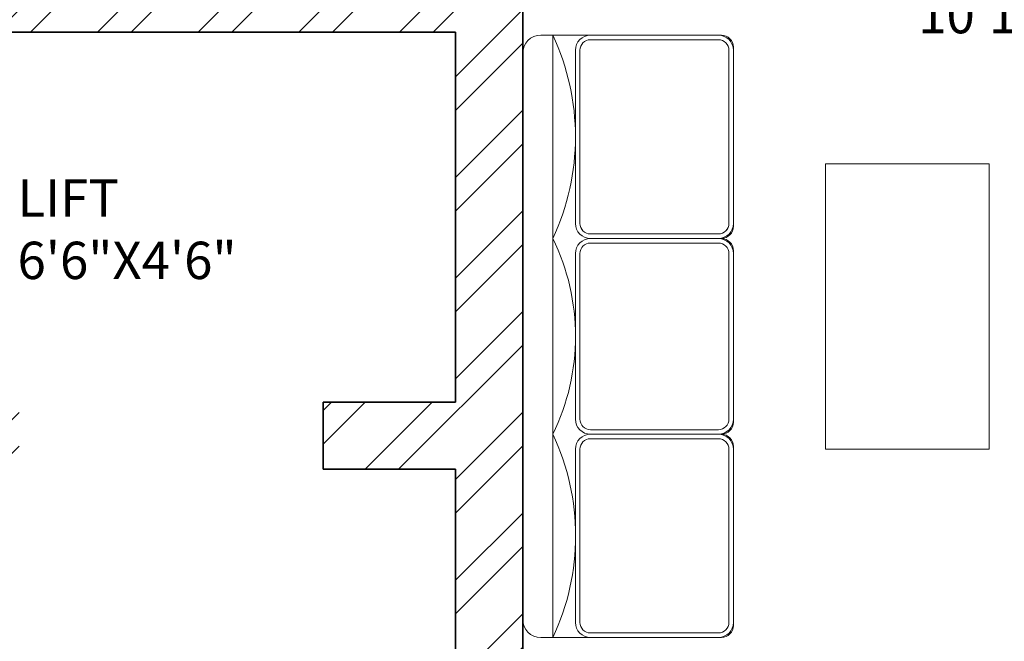
# Model space of a CAD drawing. Units: inches. Extents: x 2120 to 4013, y 1390 to 3019.
# Tile 36 of 59: x 2657 to 2789, y 2048 to 2131. Entities that reach past the tile are written whole.
import ezdxf

# ---------------------------------------------------------------- set-up
doc = ezdxf.new("R2010")
doc.units = ezdxf.units.IN
for name, color, linetype, lineweight in [('A-AREA-IDEN', 7, 'Continuous', 18), ('A-FURN', 8, 'Continuous', 13), ('A-WALL', 7, 'Continuous', 35), ('A-WALL-PATT', 252, 'Continuous', 13)]:
    doc.layers.add(name, color=color, linetype=linetype, lineweight=lineweight)
doc.styles.get("Standard").update_dxf_attribs({"font": 'arial.ttf'})

# ---------------------------------------------------------------- blocks, each defined once
blk = doc.blocks.new('TABLE-COFFEE')
blk.add_lwpolyline([(0, 38.19), (21.88, 38.19), (21.88, 0), (0, 0)], close=True)

msp = doc.modelspace()

# ---------------------------------------------------------------- hatches: boundary and pattern name
at = {"layer": 'A-WALL-PATT'}
h = msp.add_hatch(dxfattribs=at)
h.set_pattern_fill('ANSI32', color=256)
h.paths.add_polyline_path([(2271.7331, 2343.531), (2283.3788, 2343.531), (2283.3788, 2348.031), (2283.3788, 2352.5306), (2262.7331, 2352.5306), (2262.7331, 2182.638), (2267.2331, 2182.638), (2271.7331, 2182.638), (2271.7331, 2219.031), (2391.7331, 2219.031), (2391.7331, 2214.189), (2393.9831, 2214.189), (2396.2331, 2214.189), (2396.2331, 2219.031), (2420.2331, 2219.031), (2420.2331, 2225.7535), (2417.2197, 2225.7535), (2415.7331, 2225.7535), (2415.7331, 2223.5306), (2271.7331, 2223.5306)])
h.paths.add_polyline_path([(2380.0942, 2352.5306), (2343.3788, 2352.5306), (2343.3788, 2343.531), (2363.2331, 2343.531), (2363.2331, 2288.8489), (2365.4831, 2288.8489), (2367.7331, 2288.8489), (2367.7331, 2343.531), (2380.0942, 2343.531)], flags=17)
h.paths.add_polyline_path([(2432.4339, 2352.5306), (2404.0943, 2352.5306), (2404.0943, 2343.531), (2415.7331, 2343.531), (2415.7331, 2264.0306), (2367.7331, 2264.0306), (2367.7331, 2266.4872), (2363.2331, 2266.4872), (2363.2331, 2259.531), (2367.7331, 2259.531), (2415.7331, 2259.531), (2415.7331, 2255.0658), (2420.2331, 2255.0658), (2420.2331, 2259.531), (2424.5717, 2259.531), (2424.5717, 2261.781), (2424.5717, 2264.0306), (2420.2331, 2264.0306), (2420.2331, 2343.531), (2432.4339, 2343.531)])
h.paths.add_polyline_path([(2508.9115, 2352.5306), (2456.4339, 2352.5306), (2456.4339, 2343.531), (2468.2331, 2343.531), (2468.2331, 2264.0306), (2448.0487, 2264.0306), (2448.0487, 2259.531), (2468.2331, 2259.531), (2468.2331, 2255.5496), (2472.7331, 2255.5496), (2472.7331, 2343.531), (2508.9115, 2343.531)])
h.paths.add_polyline_path([(2637.7331, 2352.5306), (2544.9116, 2352.5306), (2544.9116, 2343.531), (2589.7331, 2343.531), (2633.2331, 2343.531), (2637.7331, 2343.531)])
h.paths.add_polyline_path([(2594.2331, 2343.5306), (2589.7331, 2343.5306), (2589.7331, 2259.5306), (2589.7331, 2252.4915), (2591.9831, 2252.4915), (2594.2331, 2252.4915)])
h.paths.add_polyline_path([(2637.7331, 2223.5306), (2594.2331, 2223.5306), (2594.2331, 2230.1988), (2591.9831, 2230.1988), (2589.7331, 2230.1988), (2589.7331, 2223.5306), (2472.7331, 2223.5306), (2468.2331, 2223.5306), (2468.2331, 2219.031), (2628.7331, 2219.031), (2628.7331, 2138.031), (2637.7331, 2138.031)])
h.paths.add_polyline_path([(3822.6535, 2458.4402), (3874.9468, 2458.4402), (3874.9468, 2476.9866), (3822.6535, 2476.9866)], flags=9)
h.paths.add_polyline_path([(3834.6921, 2781.8174), (3935.9206, 2781.8174), (3935.9206, 2800.3638), (3834.6921, 2800.3638)], flags=9)
h.paths.add_polyline_path([(3832.2843, 2837.9683), (3884.5776, 2837.9683), (3884.5776, 2856.5146), (3832.2843, 2856.5146)], flags=9)
h.paths.add_polyline_path([(3830.9388, 2861.4782), (3956.8958, 2861.4782), (3956.8958, 2880.0245), (3830.9388, 2880.0245)], flags=9)
h.paths.add_polyline_path([(3870.6966, 2352.5752), (3887.9272, 2352.5752), (3887.9272, 2377.3037), (3870.6966, 2377.3037)], flags=9)
h.paths.add_polyline_path([(3289.2701, 2413.161), (3435.2223, 2413.161), (3435.2223, 2450.2538), (3289.2701, 2450.2538)], flags=9)
h.paths.add_polyline_path([(2487.6944, 2414.3601), (2637.8335, 2414.3601), (2637.8335, 2451.4528), (2487.6944, 2451.4528)], flags=9)
h.paths.add_polyline_path([(2567.3724, 1457.9199), (2815.296, 1457.9199), (2815.296, 1495.0127), (2567.3724, 1495.0127)], flags=9)
h.paths.add_polyline_path([(2655.3825, 2093.2363), (2685.9555, 2093.2363), (2685.9555, 2111.8937), (2655.3825, 2111.8937)], flags=9)
h.paths.add_polyline_path([(2543.9218, 1550.6671), (2587.8406, 1550.6671), (2587.8406, 1569.3244), (2543.9218, 1569.3244)], flags=9)
h.paths.add_polyline_path([(2905.1384, 1543.8113), (2949.0572, 1543.8113), (2949.0572, 1562.4686), (2905.1384, 1562.4686)], flags=9)
h.paths.add_polyline_path([(2736.4118, 1702.4736), (2784.2153, 1702.4736), (2784.2153, 1721.1309), (2736.4118, 1721.1309)], flags=9)
h.paths.add_polyline_path([(2912.8666, 1710.4168), (2951.707, 1710.4168), (2951.707, 1729.0741), (2912.8666, 1729.0741)], flags=9)
h.paths.add_polyline_path([(2923.5785, 1763.5038), (2959.7279, 1763.5038), (2959.7279, 1782.1611), (2923.5785, 1782.1611)], flags=9)
h.paths.add_polyline_path([(2925.2114, 1809.6137), (2967.1861, 1809.6137), (2967.1861, 1828.271), (2925.2114, 1828.271)], flags=9)
h.paths.add_polyline_path([(2996.2711, 1878.9003), (2996.2711, 1913.109), (2977.6138, 1913.109), (2977.6138, 1878.9003)], flags=9)
h.paths.add_polyline_path([(2883.0859, 1895.7192), (2927.1855, 1895.7192), (2927.1855, 1914.3766), (2883.0859, 1914.3766)], flags=9)
h.paths.add_polyline_path([(2787.3924, 1810.8013), (2841.0213, 1810.8013), (2841.0213, 1829.4587), (2787.3924, 1829.4587)], flags=9)
h.paths.add_polyline_path([(2775.6399, 2101.7395), (2829.2689, 2101.7395), (2829.2689, 2120.3968), (2775.6399, 2120.3968)], flags=9)
h.paths.add_polyline_path([(2913.0263, 2075.817), (2951.8667, 2075.817), (2951.8667, 2094.4744), (2913.0263, 2094.4744)], flags=9)
h.paths.add_polyline_path([(2929.966, 2133.3669), (2966.1154, 2133.3669), (2966.1154, 2152.0243), (2929.966, 2152.0243)], flags=9)
h.paths.add_polyline_path([(2932.7502, 2182.6088), (2968.8996, 2182.6088), (2968.8996, 2201.2662), (2932.7502, 2201.2662)], flags=9)
h.paths.add_polyline_path([(2996.0681, 2266.3173), (2996.0681, 2300.5261), (2977.4108, 2300.5261), (2977.4108, 2266.3173)], flags=9)
h.paths.add_polyline_path([(2885.1039, 2279.2186), (2929.2035, 2279.2186), (2929.2035, 2297.8759), (2885.1039, 2297.8759)], flags=9)
h.paths.add_polyline_path([(2735.7042, 2218.3197), (2783.5078, 2218.3197), (2783.5078, 2236.9771), (2735.7042, 2236.9771)], flags=9)
h.paths.add_polyline_path([(2635.6049, 2044.0085), (2648.9678, 2044.0085), (2648.9678, 2054.312), (2635.6049, 2054.312)], flags=9)
h.paths.add_polyline_path([(2714.0148, 1923.0473), (2727.3777, 1923.0473), (2727.3777, 1933.3508), (2714.0148, 1933.3508)], flags=9)
h.paths.add_polyline_path([(2709.0345, 1988.1628), (2722.3974, 1988.1628), (2722.3974, 1998.4663), (2709.0345, 1998.4663)], flags=9)
h.paths.add_polyline_path([(2592.8935, 1962.1763), (2606.2564, 1962.1763), (2606.2564, 1972.4799), (2592.8935, 1972.4799)], flags=9)
h.paths.add_polyline_path([(2618.3996, 1985.9724), (2644.1942, 1985.9724), (2644.1942, 1996.2759), (2618.3996, 1996.2759)], flags=9)
h.paths.add_polyline_path([(2601.279, 1920.5869), (2614.6419, 1920.5869), (2614.6419, 1930.8904), (2601.279, 1930.8904)], flags=9)
h.paths.add_polyline_path([(2692.3278, 1932.7645), (2704.5311, 1932.7645), (2704.5311, 1943.0681), (2692.3278, 1943.0681)], flags=9)
h.paths.add_polyline_path([(2311.122, 1672.7318), (2355.0408, 1672.7318), (2355.0408, 1691.3892), (2311.122, 1691.3892)], flags=9)
h.paths.add_polyline_path([(2456.2551, 1632.3198), (2492.4796, 1632.3198), (2492.4796, 1650.9772), (2456.2551, 1650.9772)], flags=9)
h.paths.add_polyline_path([(2401.0766, 1631.4793), (2437.301, 1631.4793), (2437.301, 1650.1367), (2401.0766, 1650.1367)], flags=9)
h.paths.add_polyline_path([(2546.7054, 1700.9235), (2594.509, 1700.9235), (2594.509, 1719.5809), (2546.7054, 1719.5809)], flags=9)
h.paths.add_polyline_path([(2445.4866, 1766.9937), (2497.5261, 1766.9937), (2497.5261, 1785.651), (2445.4866, 1785.651)], flags=9)
h.paths.add_polyline_path([(2287.9992, 1739.7675), (2326.8396, 1739.7675), (2326.8396, 1758.4248), (2287.9992, 1758.4248)], flags=9)
h.paths.add_polyline_path([(2458.5279, 1924.7607), (2510.5675, 1924.7607), (2510.5675, 1943.4181), (2458.5279, 1943.4181)], flags=9)
h.paths.add_polyline_path([(2309.2811, 1902.7642), (2345.4305, 1902.7642), (2345.4305, 1921.4215), (2309.2811, 1921.4215)], flags=9)
h.paths.add_polyline_path([(2490.7554, 2018.9392), (2530.7896, 2018.9392), (2530.7896, 2037.5965), (2490.7554, 2037.5965)], flags=9)
h.paths.add_polyline_path([(2402.143, 2024.7393), (2438.5414, 2024.7393), (2438.5414, 2043.3966), (2402.143, 2043.3966)], flags=9)
h.paths.add_polyline_path([(2287.856, 1931.7926), (2326.6964, 1931.7926), (2326.6964, 1950.4499), (2287.856, 1950.4499)], flags=9)
h.paths.add_polyline_path([(2281.7979, 2193.5771), (2320.6383, 2193.5771), (2320.6383, 2212.2344), (2281.7979, 2212.2344)], flags=25)
h.paths.add_polyline_path([(2484.0754, 2093.892), (2536.115, 2093.892), (2536.115, 2112.5494), (2484.0754, 2112.5494)], flags=9)
h.paths.add_polyline_path([(2624.7948, 2281.8639), (2624.7948, 2311.4137), (2606.1375, 2311.4137), (2606.1375, 2281.8639)], flags=9)
h.paths.add_polyline_path([(2507.5036, 2290.3639), (2541.934, 2290.3639), (2541.934, 2309.0212), (2507.5036, 2309.0212)], flags=9)
h.paths.add_polyline_path([(2423.1076, 2285.2202), (2459.332, 2285.2202), (2459.332, 2303.8776), (2423.1076, 2303.8776)], flags=9)
h.paths.add_polyline_path([(2374.5467, 2289.6272), (2410.7711, 2289.6272), (2410.7711, 2308.2846), (2374.5467, 2308.2846)], flags=25)
h.paths.add_polyline_path([(2277.4907, 2227.5651), (2316.3311, 2227.5651), (2316.3311, 2246.2224), (2277.4907, 2246.2224)], flags=25)
h.paths.add_polyline_path([(2655.3825, 2093.2367), (2685.9555, 2093.2367), (2685.9555, 2111.894), (2655.3825, 2111.894)], flags=9)
h.paths.add_polyline_path([(2543.9217, 1550.6674), (2587.8406, 1550.6674), (2587.8406, 1569.3247), (2543.9217, 1569.3247)], flags=9)
h.paths.add_polyline_path([(2905.1384, 1543.8116), (2949.0572, 1543.8116), (2949.0572, 1562.4689), (2905.1384, 1562.4689)], flags=9)
h.paths.add_polyline_path([(2736.4118, 1702.4739), (2784.2153, 1702.4739), (2784.2153, 1721.1312), (2736.4118, 1721.1312)], flags=9)
h.paths.add_polyline_path([(2912.8666, 1710.4171), (2951.707, 1710.4171), (2951.707, 1729.0744), (2912.8666, 1729.0744)], flags=9)
h.paths.add_polyline_path([(2923.5785, 1763.5041), (2959.7279, 1763.5041), (2959.7279, 1782.1614), (2923.5785, 1782.1614)], flags=9)
h.paths.add_polyline_path([(2925.2114, 1809.614), (2967.1861, 1809.614), (2967.1861, 1828.2713), (2925.2114, 1828.2713)], flags=9)
h.paths.add_polyline_path([(2996.2711, 1878.9006), (2996.2711, 1913.1094), (2977.6137, 1913.1094), (2977.6137, 1878.9006)], flags=9)
h.paths.add_polyline_path([(2883.0859, 1895.7195), (2927.1855, 1895.7195), (2927.1855, 1914.3769), (2883.0859, 1914.3769)], flags=9)
h.paths.add_polyline_path([(2787.3924, 1810.8016), (2841.0213, 1810.8016), (2841.0213, 1829.459), (2787.3924, 1829.459)], flags=9)
h.paths.add_polyline_path([(2775.6399, 2101.7398), (2829.2688, 2101.7398), (2829.2688, 2120.3971), (2775.6399, 2120.3971)], flags=9)
h.paths.add_polyline_path([(2913.0263, 2075.8173), (2951.8667, 2075.8173), (2951.8667, 2094.4747), (2913.0263, 2094.4747)], flags=9)
h.paths.add_polyline_path([(2929.966, 2133.3672), (2966.1154, 2133.3672), (2966.1154, 2152.0246), (2929.966, 2152.0246)], flags=9)
h.paths.add_polyline_path([(2932.7502, 2182.6091), (2968.8996, 2182.6091), (2968.8996, 2201.2665), (2932.7502, 2201.2665)], flags=9)
h.paths.add_polyline_path([(2996.0681, 2266.3176), (2996.0681, 2300.5264), (2977.4108, 2300.5264), (2977.4108, 2266.3176)], flags=9)
h.paths.add_polyline_path([(2885.1039, 2279.2189), (2929.2035, 2279.2189), (2929.2035, 2297.8762), (2885.1039, 2297.8762)], flags=9)
h.paths.add_polyline_path([(2735.7042, 2218.32), (2783.5078, 2218.32), (2783.5078, 2236.9774), (2735.7042, 2236.9774)], flags=9)
h.paths.add_polyline_path([(2635.6048, 2044.0088), (2648.9677, 2044.0088), (2648.9677, 2054.3123), (2635.6048, 2054.3123)], flags=9)
h.paths.add_polyline_path([(2714.0148, 1923.0476), (2727.3777, 1923.0476), (2727.3777, 1933.3511), (2714.0148, 1933.3511)], flags=9)
h.paths.add_polyline_path([(2709.0345, 1988.1631), (2722.3974, 1988.1631), (2722.3974, 1998.4666), (2709.0345, 1998.4666)], flags=9)
h.paths.add_polyline_path([(2592.8935, 1962.1766), (2606.2564, 1962.1766), (2606.2564, 1972.4802), (2592.8935, 1972.4802)], flags=9)
h.paths.add_polyline_path([(2618.3995, 1985.9727), (2644.1942, 1985.9727), (2644.1942, 1996.2762), (2618.3995, 1996.2762)], flags=9)
h.paths.add_polyline_path([(2601.279, 1920.5872), (2614.6419, 1920.5872), (2614.6419, 1930.8908), (2601.279, 1930.8908)], flags=9)
h.paths.add_polyline_path([(2692.3278, 1932.7648), (2704.5311, 1932.7648), (2704.5311, 1943.0684), (2692.3278, 1943.0684)], flags=9)
h.paths.add_polyline_path([(2311.122, 1672.7321), (2355.0408, 1672.7321), (2355.0408, 1691.3895), (2311.122, 1691.3895)], flags=9)
h.paths.add_polyline_path([(2456.2551, 1632.3201), (2492.4795, 1632.3201), (2492.4795, 1650.9775), (2456.2551, 1650.9775)], flags=9)
h.paths.add_polyline_path([(2401.0766, 1631.4796), (2437.301, 1631.4796), (2437.301, 1650.137), (2401.0766, 1650.137)], flags=9)
h.paths.add_polyline_path([(2546.7054, 1700.9238), (2594.509, 1700.9238), (2594.509, 1719.5812), (2546.7054, 1719.5812)], flags=9)
h.paths.add_polyline_path([(2445.4866, 1766.994), (2497.5261, 1766.994), (2497.5261, 1785.6513), (2445.4866, 1785.6513)], flags=9)
h.paths.add_polyline_path([(2287.9992, 1739.7678), (2326.8396, 1739.7678), (2326.8396, 1758.4251), (2287.9992, 1758.4251)], flags=9)
h.paths.add_polyline_path([(2458.5279, 1924.7611), (2510.5675, 1924.7611), (2510.5675, 1943.4184), (2458.5279, 1943.4184)], flags=9)
h.paths.add_polyline_path([(2309.2811, 1902.7645), (2345.4305, 1902.7645), (2345.4305, 1921.4218), (2309.2811, 1921.4218)], flags=9)
h.paths.add_polyline_path([(2490.7554, 2018.9395), (2530.7895, 2018.9395), (2530.7895, 2037.5968), (2490.7554, 2037.5968)], flags=9)
h.paths.add_polyline_path([(2402.143, 2024.7396), (2438.5413, 2024.7396), (2438.5413, 2043.3969), (2402.143, 2043.3969)], flags=9)
h.paths.add_polyline_path([(2287.856, 1931.7929), (2326.6964, 1931.7929), (2326.6964, 1950.4502), (2287.856, 1950.4502)], flags=9)
h.paths.add_polyline_path([(2281.7979, 2193.5774), (2320.6383, 2193.5774), (2320.6383, 2212.2347), (2281.7979, 2212.2347)], flags=25)
h.paths.add_polyline_path([(2484.0754, 2093.8924), (2536.115, 2093.8924), (2536.115, 2112.5497), (2484.0754, 2112.5497)], flags=9)
h.paths.add_polyline_path([(2624.7948, 2281.8642), (2624.7948, 2311.414), (2606.1374, 2311.414), (2606.1374, 2281.8642)], flags=9)
h.paths.add_polyline_path([(2507.5035, 2290.3642), (2541.934, 2290.3642), (2541.934, 2309.0215), (2507.5035, 2309.0215)], flags=9)
h.paths.add_polyline_path([(2423.1075, 2285.2205), (2459.332, 2285.2205), (2459.332, 2303.8779), (2423.1075, 2303.8779)], flags=9)
h.paths.add_polyline_path([(2374.5467, 2289.6275), (2410.7711, 2289.6275), (2410.7711, 2308.2849), (2374.5467, 2308.2849)], flags=25)
h.paths.add_polyline_path([(2277.4907, 2227.5654), (2316.3311, 2227.5654), (2316.3311, 2246.2227), (2277.4907, 2246.2227)], flags=25)
h = msp.add_hatch(dxfattribs=at)
h.set_pattern_fill('ANSI32', color=256)
h.paths.add_polyline_path([(2271.7331, 1980.389), (2262.7331, 1980.389), (2262.7331, 1912.8434), (2267.2331, 1912.8434), (2271.7331, 1912.8434), (2271.7331, 1922.531), (2351.2331, 1922.531), (2351.2331, 1901.4728), (2355.7331, 1901.4728), (2355.7331, 1922.531), (2357.9815, 1922.531), (2357.9815, 1926.5306), (2271.7331, 1926.5306)])
h.paths.add_polyline_path([(2589.2331, 1949.1622), (2584.7331, 1949.1622), (2580.2331, 1949.1622), (2580.2331, 1874.5306), (2355.7331, 1874.5306), (2355.7331, 1880.1922), (2351.2331, 1880.1922), (2351.2331, 1874.5306), (2271.7331, 1874.5306), (2271.7331, 1888.8431), (2262.7331, 1888.8431), (2262.7331, 1842.2909), (2267.2331, 1842.2909), (2271.7331, 1842.2909), (2271.7331, 1865.531), (2415.7331, 1865.531), (2415.7331, 1779.7286), (2420.2331, 1779.7286), (2420.2331, 1865.531), (2589.2331, 1865.531)])
h.paths.add_polyline_path([(2271.7331, 1782.2906), (2262.7331, 1782.2906), (2262.7331, 1711.4639), (2267.2331, 1711.4639), (2271.7331, 1711.4639), (2271.7331, 1738.031), (2420.2331, 1738.031), (2420.2331, 1742.531), (2420.2331, 1747.3376), (2417.9831, 1747.3376), (2415.7331, 1747.3376), (2415.7331, 1742.5306), (2271.7331, 1742.5306)])
h.paths.add_polyline_path([(2271.7331, 1627.031), (2362.3957, 1627.031), (2362.3957, 1629.281), (2362.3957, 1631.5306), (2271.7331, 1631.5306), (2271.7331, 1675.4636), (2262.7331, 1675.4636), (2262.7331, 1581.531), (2405.3032, 1581.531), (2405.3032, 1586.031), (2405.3032, 1590.5306), (2396.2331, 1590.5306), (2396.2331, 1691.4513), (2418.7206, 1691.4513), (2418.7206, 1695.951), (2396.2331, 1695.951), (2391.7331, 1695.951), (2391.7331, 1631.5306), (2386.7425, 1631.5306), (2386.7425, 1629.2806), (2386.7425, 1627.031), (2391.7331, 1627.031), (2391.7331, 1586.1709), (2271.7331, 1586.1709)])
h.paths.add_polyline_path([(2459.6703, 1590.5306), (2429.3032, 1590.5306), (2429.3032, 1581.531), (2459.6703, 1581.531), (2459.6703, 1586.031)])
h.paths.add_polyline_path([(2501.2331, 1590.531), (2501.2331, 1665.0195), (2498.9831, 1665.0195), (2496.7331, 1665.0195), (2496.7331, 1590.5306), (2483.8201, 1590.5306), (2483.8201, 1590.1579), (2483.6704, 1590.1579), (2483.6704, 1581.531), (2505.0196, 1581.531), (2505.0196, 1583.781), (2505.0196, 1586.0306), (2501.2331, 1586.0306)])
h.paths.add_polyline_path([(2544.1361, 1583.781), (2544.1361, 1586.0306), (2527.1368, 1586.0306), (2527.1368, 1583.7806), (2527.1368, 1581.531), (2544.1361, 1581.531)])
h.paths.add_polyline_path([(3822.6535, 2458.4402), (3874.9468, 2458.4402), (3874.9468, 2476.9866), (3822.6535, 2476.9866)], flags=9)
h.paths.add_polyline_path([(3834.6921, 2781.8174), (3935.9206, 2781.8174), (3935.9206, 2800.3638), (3834.6921, 2800.3638)], flags=9)
h.paths.add_polyline_path([(3832.2843, 2837.9683), (3884.5776, 2837.9683), (3884.5776, 2856.5146), (3832.2843, 2856.5146)], flags=9)
h.paths.add_polyline_path([(3830.9388, 2861.4782), (3956.8958, 2861.4782), (3956.8958, 2880.0245), (3830.9388, 2880.0245)], flags=9)
h.paths.add_polyline_path([(3870.6966, 2352.5752), (3887.9272, 2352.5752), (3887.9272, 2377.3037), (3870.6966, 2377.3037)], flags=9)
h.paths.add_polyline_path([(3289.2701, 2413.161), (3435.2223, 2413.161), (3435.2223, 2450.2538), (3289.2701, 2450.2538)], flags=9)
h.paths.add_polyline_path([(2487.6944, 2414.3601), (2637.8335, 2414.3601), (2637.8335, 2451.4528), (2487.6944, 2451.4528)], flags=9)
h.paths.add_polyline_path([(2567.3724, 1457.9199), (2815.296, 1457.9199), (2815.296, 1495.0127), (2567.3724, 1495.0127)], flags=9)
h.paths.add_polyline_path([(2655.3825, 2093.2363), (2685.9555, 2093.2363), (2685.9555, 2111.8937), (2655.3825, 2111.8937)], flags=9)
h.paths.add_polyline_path([(2543.9218, 1550.6671), (2587.8406, 1550.6671), (2587.8406, 1569.3244), (2543.9218, 1569.3244)], flags=9)
h.paths.add_polyline_path([(2905.1384, 1543.8113), (2949.0572, 1543.8113), (2949.0572, 1562.4686), (2905.1384, 1562.4686)], flags=9)
h.paths.add_polyline_path([(2736.4118, 1702.4736), (2784.2153, 1702.4736), (2784.2153, 1721.1309), (2736.4118, 1721.1309)], flags=9)
h.paths.add_polyline_path([(2912.8666, 1710.4168), (2951.707, 1710.4168), (2951.707, 1729.0741), (2912.8666, 1729.0741)], flags=9)
h.paths.add_polyline_path([(2923.5785, 1763.5038), (2959.7279, 1763.5038), (2959.7279, 1782.1611), (2923.5785, 1782.1611)], flags=9)
h.paths.add_polyline_path([(2925.2114, 1809.6137), (2967.1861, 1809.6137), (2967.1861, 1828.271), (2925.2114, 1828.271)], flags=9)
h.paths.add_polyline_path([(2996.2711, 1878.9003), (2996.2711, 1913.109), (2977.6138, 1913.109), (2977.6138, 1878.9003)], flags=9)
h.paths.add_polyline_path([(2883.0859, 1895.7192), (2927.1855, 1895.7192), (2927.1855, 1914.3766), (2883.0859, 1914.3766)], flags=9)
h.paths.add_polyline_path([(2787.3924, 1810.8013), (2841.0213, 1810.8013), (2841.0213, 1829.4587), (2787.3924, 1829.4587)], flags=9)
h.paths.add_polyline_path([(2775.6399, 2101.7395), (2829.2689, 2101.7395), (2829.2689, 2120.3968), (2775.6399, 2120.3968)], flags=9)
h.paths.add_polyline_path([(2913.0263, 2075.817), (2951.8667, 2075.817), (2951.8667, 2094.4744), (2913.0263, 2094.4744)], flags=9)
h.paths.add_polyline_path([(2929.966, 2133.3669), (2966.1154, 2133.3669), (2966.1154, 2152.0243), (2929.966, 2152.0243)], flags=9)
h.paths.add_polyline_path([(2932.7502, 2182.6088), (2968.8996, 2182.6088), (2968.8996, 2201.2662), (2932.7502, 2201.2662)], flags=9)
h.paths.add_polyline_path([(2996.0681, 2266.3173), (2996.0681, 2300.5261), (2977.4108, 2300.5261), (2977.4108, 2266.3173)], flags=9)
h.paths.add_polyline_path([(2885.1039, 2279.2186), (2929.2035, 2279.2186), (2929.2035, 2297.8759), (2885.1039, 2297.8759)], flags=9)
h.paths.add_polyline_path([(2735.7042, 2218.3197), (2783.5078, 2218.3197), (2783.5078, 2236.9771), (2735.7042, 2236.9771)], flags=9)
h.paths.add_polyline_path([(2635.6049, 2044.0085), (2648.9678, 2044.0085), (2648.9678, 2054.312), (2635.6049, 2054.312)], flags=9)
h.paths.add_polyline_path([(2714.0148, 1923.0473), (2727.3777, 1923.0473), (2727.3777, 1933.3508), (2714.0148, 1933.3508)], flags=9)
h.paths.add_polyline_path([(2709.0345, 1988.1628), (2722.3974, 1988.1628), (2722.3974, 1998.4663), (2709.0345, 1998.4663)], flags=9)
h.paths.add_polyline_path([(2592.8935, 1962.1763), (2606.2564, 1962.1763), (2606.2564, 1972.4799), (2592.8935, 1972.4799)], flags=9)
h.paths.add_polyline_path([(2618.3996, 1985.9724), (2644.1942, 1985.9724), (2644.1942, 1996.2759), (2618.3996, 1996.2759)], flags=9)
h.paths.add_polyline_path([(2601.279, 1920.5869), (2614.6419, 1920.5869), (2614.6419, 1930.8904), (2601.279, 1930.8904)], flags=9)
h.paths.add_polyline_path([(2692.3278, 1932.7645), (2704.5311, 1932.7645), (2704.5311, 1943.0681), (2692.3278, 1943.0681)], flags=9)
h.paths.add_polyline_path([(2311.122, 1672.7318), (2355.0408, 1672.7318), (2355.0408, 1691.3892), (2311.122, 1691.3892)], flags=25)
h.paths.add_polyline_path([(2456.2551, 1632.3198), (2492.4796, 1632.3198), (2492.4796, 1650.9772), (2456.2551, 1650.9772)], flags=9)
h.paths.add_polyline_path([(2401.0766, 1631.4793), (2437.301, 1631.4793), (2437.301, 1650.1367), (2401.0766, 1650.1367)], flags=9)
h.paths.add_polyline_path([(2546.7054, 1700.9235), (2594.509, 1700.9235), (2594.509, 1719.5809), (2546.7054, 1719.5809)], flags=9)
h.paths.add_polyline_path([(2445.4866, 1766.9937), (2497.5261, 1766.9937), (2497.5261, 1785.651), (2445.4866, 1785.651)], flags=9)
h.paths.add_polyline_path([(2287.9992, 1739.7675), (2326.8396, 1739.7675), (2326.8396, 1758.4248), (2287.9992, 1758.4248)], flags=24)
h.paths.add_polyline_path([(2458.5279, 1924.7607), (2510.5675, 1924.7607), (2510.5675, 1943.4181), (2458.5279, 1943.4181)], flags=25)
h.paths.add_polyline_path([(2309.2811, 1902.7642), (2345.4305, 1902.7642), (2345.4305, 1921.4215), (2309.2811, 1921.4215)], flags=25)
h.paths.add_polyline_path([(2490.7554, 2018.9392), (2530.7896, 2018.9392), (2530.7896, 2037.5965), (2490.7554, 2037.5965)], flags=9)
h.paths.add_polyline_path([(2402.143, 2024.7393), (2438.5414, 2024.7393), (2438.5414, 2043.3966), (2402.143, 2043.3966)], flags=9)
h.paths.add_polyline_path([(2287.856, 1931.7926), (2326.6964, 1931.7926), (2326.6964, 1950.4499), (2287.856, 1950.4499)], flags=25)
h.paths.add_polyline_path([(2281.7979, 2193.5771), (2320.6383, 2193.5771), (2320.6383, 2212.2344), (2281.7979, 2212.2344)], flags=9)
h.paths.add_polyline_path([(2484.0754, 2093.892), (2536.115, 2093.892), (2536.115, 2112.5494), (2484.0754, 2112.5494)], flags=9)
h.paths.add_polyline_path([(2624.7948, 2281.8639), (2624.7948, 2311.4137), (2606.1375, 2311.4137), (2606.1375, 2281.8639)], flags=9)
h.paths.add_polyline_path([(2507.5036, 2290.3639), (2541.934, 2290.3639), (2541.934, 2309.0212), (2507.5036, 2309.0212)], flags=9)
h.paths.add_polyline_path([(2423.1076, 2285.2202), (2459.332, 2285.2202), (2459.332, 2303.8776), (2423.1076, 2303.8776)], flags=9)
h.paths.add_polyline_path([(2374.5467, 2289.6272), (2410.7711, 2289.6272), (2410.7711, 2308.2846), (2374.5467, 2308.2846)], flags=9)
h.paths.add_polyline_path([(2277.4907, 2227.5651), (2316.3311, 2227.5651), (2316.3311, 2246.2224), (2277.4907, 2246.2224)], flags=9)
h.paths.add_polyline_path([(2655.3825, 2093.2367), (2685.9555, 2093.2367), (2685.9555, 2111.894), (2655.3825, 2111.894)], flags=9)
h.paths.add_polyline_path([(2543.9217, 1550.6674), (2587.8406, 1550.6674), (2587.8406, 1569.3247), (2543.9217, 1569.3247)], flags=9)
h.paths.add_polyline_path([(2905.1384, 1543.8116), (2949.0572, 1543.8116), (2949.0572, 1562.4689), (2905.1384, 1562.4689)], flags=9)
h.paths.add_polyline_path([(2736.4118, 1702.4739), (2784.2153, 1702.4739), (2784.2153, 1721.1312), (2736.4118, 1721.1312)], flags=9)
h.paths.add_polyline_path([(2912.8666, 1710.4171), (2951.707, 1710.4171), (2951.707, 1729.0744), (2912.8666, 1729.0744)], flags=9)
h.paths.add_polyline_path([(2923.5785, 1763.5041), (2959.7279, 1763.5041), (2959.7279, 1782.1614), (2923.5785, 1782.1614)], flags=9)
h.paths.add_polyline_path([(2925.2114, 1809.614), (2967.1861, 1809.614), (2967.1861, 1828.2713), (2925.2114, 1828.2713)], flags=9)
h.paths.add_polyline_path([(2996.2711, 1878.9006), (2996.2711, 1913.1094), (2977.6137, 1913.1094), (2977.6137, 1878.9006)], flags=9)
h.paths.add_polyline_path([(2883.0859, 1895.7195), (2927.1855, 1895.7195), (2927.1855, 1914.3769), (2883.0859, 1914.3769)], flags=9)
h.paths.add_polyline_path([(2787.3924, 1810.8016), (2841.0213, 1810.8016), (2841.0213, 1829.459), (2787.3924, 1829.459)], flags=9)
h.paths.add_polyline_path([(2775.6399, 2101.7398), (2829.2688, 2101.7398), (2829.2688, 2120.3971), (2775.6399, 2120.3971)], flags=9)
h.paths.add_polyline_path([(2913.0263, 2075.8173), (2951.8667, 2075.8173), (2951.8667, 2094.4747), (2913.0263, 2094.4747)], flags=9)
h.paths.add_polyline_path([(2929.966, 2133.3672), (2966.1154, 2133.3672), (2966.1154, 2152.0246), (2929.966, 2152.0246)], flags=9)
h.paths.add_polyline_path([(2932.7502, 2182.6091), (2968.8996, 2182.6091), (2968.8996, 2201.2665), (2932.7502, 2201.2665)], flags=9)
h.paths.add_polyline_path([(2996.0681, 2266.3176), (2996.0681, 2300.5264), (2977.4108, 2300.5264), (2977.4108, 2266.3176)], flags=9)
h.paths.add_polyline_path([(2885.1039, 2279.2189), (2929.2035, 2279.2189), (2929.2035, 2297.8762), (2885.1039, 2297.8762)], flags=9)
h.paths.add_polyline_path([(2735.7042, 2218.32), (2783.5078, 2218.32), (2783.5078, 2236.9774), (2735.7042, 2236.9774)], flags=9)
h.paths.add_polyline_path([(2635.6048, 2044.0088), (2648.9677, 2044.0088), (2648.9677, 2054.3123), (2635.6048, 2054.3123)], flags=9)
h.paths.add_polyline_path([(2714.0148, 1923.0476), (2727.3777, 1923.0476), (2727.3777, 1933.3511), (2714.0148, 1933.3511)], flags=9)
h.paths.add_polyline_path([(2709.0345, 1988.1631), (2722.3974, 1988.1631), (2722.3974, 1998.4666), (2709.0345, 1998.4666)], flags=9)
h.paths.add_polyline_path([(2592.8935, 1962.1766), (2606.2564, 1962.1766), (2606.2564, 1972.4802), (2592.8935, 1972.4802)], flags=9)
h.paths.add_polyline_path([(2618.3995, 1985.9727), (2644.1942, 1985.9727), (2644.1942, 1996.2762), (2618.3995, 1996.2762)], flags=9)
h.paths.add_polyline_path([(2601.279, 1920.5872), (2614.6419, 1920.5872), (2614.6419, 1930.8908), (2601.279, 1930.8908)], flags=9)
h.paths.add_polyline_path([(2692.3278, 1932.7648), (2704.5311, 1932.7648), (2704.5311, 1943.0684), (2692.3278, 1943.0684)], flags=9)
h.paths.add_polyline_path([(2311.122, 1672.7321), (2355.0408, 1672.7321), (2355.0408, 1691.3895), (2311.122, 1691.3895)], flags=25)
h.paths.add_polyline_path([(2456.2551, 1632.3201), (2492.4795, 1632.3201), (2492.4795, 1650.9775), (2456.2551, 1650.9775)], flags=9)
h.paths.add_polyline_path([(2401.0766, 1631.4796), (2437.301, 1631.4796), (2437.301, 1650.137), (2401.0766, 1650.137)], flags=9)
h.paths.add_polyline_path([(2546.7054, 1700.9238), (2594.509, 1700.9238), (2594.509, 1719.5812), (2546.7054, 1719.5812)], flags=9)
h.paths.add_polyline_path([(2445.4866, 1766.994), (2497.5261, 1766.994), (2497.5261, 1785.6513), (2445.4866, 1785.6513)], flags=9)
h.paths.add_polyline_path([(2287.9992, 1739.7678), (2326.8396, 1739.7678), (2326.8396, 1758.4251), (2287.9992, 1758.4251)], flags=24)
h.paths.add_polyline_path([(2458.5279, 1924.7611), (2510.5675, 1924.7611), (2510.5675, 1943.4184), (2458.5279, 1943.4184)], flags=25)
h.paths.add_polyline_path([(2309.2811, 1902.7645), (2345.4305, 1902.7645), (2345.4305, 1921.4218), (2309.2811, 1921.4218)], flags=25)
h.paths.add_polyline_path([(2490.7554, 2018.9395), (2530.7895, 2018.9395), (2530.7895, 2037.5968), (2490.7554, 2037.5968)], flags=9)
h.paths.add_polyline_path([(2402.143, 2024.7396), (2438.5413, 2024.7396), (2438.5413, 2043.3969), (2402.143, 2043.3969)], flags=9)
h.paths.add_polyline_path([(2287.856, 1931.7929), (2326.6964, 1931.7929), (2326.6964, 1950.4502), (2287.856, 1950.4502)], flags=25)
h.paths.add_polyline_path([(2281.7979, 2193.5774), (2320.6383, 2193.5774), (2320.6383, 2212.2347), (2281.7979, 2212.2347)], flags=9)
h.paths.add_polyline_path([(2484.0754, 2093.8924), (2536.115, 2093.8924), (2536.115, 2112.5497), (2484.0754, 2112.5497)], flags=9)
h.paths.add_polyline_path([(2624.7948, 2281.8642), (2624.7948, 2311.414), (2606.1374, 2311.414), (2606.1374, 2281.8642)], flags=9)
h.paths.add_polyline_path([(2507.5035, 2290.3642), (2541.934, 2290.3642), (2541.934, 2309.0215), (2507.5035, 2309.0215)], flags=9)
h.paths.add_polyline_path([(2423.1075, 2285.2205), (2459.332, 2285.2205), (2459.332, 2303.8779), (2423.1075, 2303.8779)], flags=9)
h.paths.add_polyline_path([(2374.5467, 2289.6275), (2410.7711, 2289.6275), (2410.7711, 2308.2849), (2374.5467, 2308.2849)], flags=9)
h.paths.add_polyline_path([(2277.4907, 2227.5654), (2316.3311, 2227.5654), (2316.3311, 2246.2227), (2277.4907, 2246.2227)], flags=9)
h = msp.add_hatch(dxfattribs=at)
h.set_pattern_fill('ANSI32', color=256)
h.paths.add_polyline_path([(2271.7331, 2122.6377), (2262.7331, 2122.6377), (2262.7331, 2040.3893), (2267.2331, 2040.3893), (2271.7331, 2040.3893), (2271.7331, 2044.8856), (2271.7331, 2070.531), (2391.7331, 2070.531), (2391.7331, 1926.5306), (2388.3993, 1926.5306), (2388.3993, 1922.531), (2395.7331, 1922.531), (2395.7331, 1992.531), (2400.4511, 1992.531), (2400.4511, 1997.0306), (2395.7331, 1997.0306), (2395.7331, 2070.531), (2443.7331, 2070.531), (2443.7331, 2046.1368), (2448.2331, 2046.1368), (2448.2331, 2070.531), (2580.2331, 2070.531), (2580.2331, 1997.0306), (2492.9076, 1997.0306), (2492.9076, 1992.531), (2580.2331, 1992.531), (2580.2331, 1983.9368), (2589.2331, 1983.9368), (2589.2331, 2070.531), (2589.2331, 2075.0306), (2396.2331, 2075.0306), (2396.2331, 2184.3565), (2393.9831, 2184.3565), (2391.7331, 2184.3565), (2391.7331, 2075.0306), (2271.7331, 2075.0306)])
h.paths.add_polyline_path([(2724.7331, 2138.0306), (2628.7331, 2138.0306), (2628.7331, 2070.5306), (2628.7331, 2067.0987), (2633.2331, 2067.0987), (2637.7331, 2067.0987), (2637.7331, 2070.531), (2657.3413, 2070.531), (2657.3413, 2079.5306), (2637.7331, 2079.5306), (2637.7331, 2129.031), (2715.7331, 2129.031), (2715.7331, 2079.5306), (2698.0378, 2079.5306), (2698.0378, 2070.531), (2715.7331, 2070.531), (2715.7331, 2012.1531), (2720.2331, 2012.1531), (2724.7331, 2012.1531)])
h.paths.add_polyline_path([(2724.7331, 2213.031), (2831.3209, 2213.031), (2831.3209, 2215.281), (2831.3209, 2217.5306), (2724.7331, 2217.5306), (2724.7331, 2343.531), (2751.8755, 2343.531), (2751.8755, 2352.5306), (2715.7331, 2352.5306), (2715.7331, 2138.031), (2724.7331, 2138.031)])
h.paths.add_polyline_path([(2902.53, 2352.5306), (2811.8755, 2352.5306), (2811.8755, 2343.531), (2867.2331, 2343.531), (2867.2331, 2217.5306), (2863.6364, 2217.5306), (2863.6364, 2213.031), (2871.7331, 2213.031), (2871.7331, 2217.531), (2871.7331, 2343.531), (2902.53, 2343.531)])
h.paths.add_polyline_path([(3009.7331, 2352.5306), (2938.53, 2352.5306), (2938.53, 2343.531), (2966.2331, 2343.531), (2966.2331, 2242.3281), (2968.4831, 2242.3281), (2970.7331, 2242.3281), (2970.7331, 2343.531), (3009.7331, 2343.531)])
h.paths.add_polyline_path([(3009.7331, 2217.5306), (2970.7331, 2217.5306), (2970.7331, 2220.5422), (2968.4831, 2220.5422), (2966.2331, 2220.5422), (2966.2331, 2217.5306), (2911.7752, 2217.5306), (2907.7331, 2217.5306), (2907.7331, 2213.0306), (2907.7331, 2194.9663), (2912.2331, 2194.9663), (2912.2331, 2213.031), (2970.7331, 2213.031), (3000.7331, 2213.031), (3000.7331, 2205.523), (3009.7331, 2205.523)])
h.paths.add_polyline_path([(3009.7331, 2181.5227), (3000.7331, 2181.5227), (3000.7331, 2165.0306), (2912.2331, 2165.0306), (2912.2331, 2170.8202), (2907.7331, 2170.8202), (2907.7331, 2165.0306), (2899.5169, 2165.0306), (2899.5169, 2162.7806), (2899.5169, 2160.531), (2907.7331, 2160.531), (2907.7331, 2137.3432), (2912.2331, 2137.3432), (2912.2331, 2160.531), (3000.7331, 2160.531), (3000.7331, 2150.4993), (3009.7331, 2150.4993)])
h.paths.add_polyline_path([(3009.7331, 2126.499), (3005.2331, 2126.499), (3000.7331, 2126.499), (3000.7331, 2112.5306), (2912.2331, 2112.5306), (2912.2331, 2115.6036), (2907.7331, 2115.6036), (2907.7331, 2108.031), (3000.7331, 2108.031), (3000.7331, 2084.7256), (3009.7331, 2084.7256)], flags=17)
h.paths.add_polyline_path([(3009.7331, 1971.531), (3009.7331, 2024.7253), (3000.7331, 2024.7253), (3000.7331, 2006.4153), (3000.7331, 1971.5306), (2864.2331, 1971.5306), (2864.2331, 2160.531), (2868.0522, 2160.531), (2868.0522, 2165.0306), (2859.7331, 2165.0306), (2859.7331, 1971.5306), (2724.7331, 1971.5306), (2724.7331, 1977.7012), (2715.7331, 1977.7012), (2715.7331, 1962.5306), (2715.7331, 1950.9035), (2720.2331, 1950.9035), (2724.7331, 1950.9035), (2724.7331, 1962.531), (2855.2331, 1962.531), (2859.7331, 1962.531), (2859.7331, 1835.031), (2864.2331, 1834.8158), (2864.2331, 1962.531), (2958.7331, 1962.531), (2958.7331, 1937.0925), (2963.2331, 1937.0925), (2963.2331, 1962.531), (3000.7331, 1962.531), (3009.7331, 1962.531)])
h.paths.add_polyline_path([(2724.7331, 1728.531), (2822.7164, 1728.531), (2822.7164, 1733.0306), (2724.7331, 1733.0306), (2724.7331, 1779.3416), (2715.7331, 1779.3416), (2715.7331, 1581.531), (2753.02, 1581.531), (2753.02, 1586.031), (2753.02, 1590.5306), (2724.7331, 1590.5306)])
h.paths.add_polyline_path([(2864.2331, 1590.531), (2864.2331, 1787.031), (2868.4075, 1787.031), (2868.4075, 1791.5306), (2859.7331, 1791.5306), (2859.7331, 1739.0306), (2859.7331, 1733.0306), (2854.3125, 1733.0306), (2854.3125, 1728.531), (2859.7331, 1728.531), (2859.7331, 1590.5306), (2813.02, 1590.5306), (2813.02, 1581.531), (2868.4123, 1581.531), (2868.4123, 1583.781), (2868.4123, 1586.0306), (2864.2331, 1586.0306)])
h.paths.add_polyline_path([(3009.7331, 1754.6619), (3000.7331, 1754.6619), (3000.7331, 1739.0306), (2912.2331, 1739.0306), (2912.2331, 1742.2257), (2907.7331, 1742.2257), (2907.7331, 1739.0306), (2907.7331, 1734.531), (3000.7331, 1734.531), (3000.7331, 1590.5306), (3000.7331, 1586.0306), (2971.3921, 1586.0306), (2971.3921, 1581.531), (3009.7331, 1581.531)])
h.paths.add_polyline_path([(2911.3921, 1583.781), (2911.3921, 1586.0306), (2891.2138, 1586.0306), (2891.2138, 1581.531), (2911.3921, 1581.531)])
h.paths.add_polyline_path([(3009.7331, 1799.8422), (3000.7331, 1799.8422), (3000.7331, 1791.5306), (2912.2331, 1791.5306), (2912.2331, 1796.3264), (2909.9831, 1796.3264), (2907.7331, 1796.3264), (2907.7331, 1791.5306), (2902.7033, 1791.5306), (2902.7033, 1787.031), (2907.7331, 1787.031), (2907.7331, 1761.1622), (2912.2331, 1761.1622), (2912.2331, 1787.031), (3000.7331, 1787.031), (3000.7331, 1778.6622), (3009.7331, 1778.6622)])
h.paths.add_polyline_path([(3009.7331, 1839.5306), (2963.2331, 1839.5306), (2963.2331, 1842.8629), (2960.9831, 1842.8629), (2958.7331, 1842.8629), (2958.7331, 1839.5306), (2907.7331, 1839.5306), (2907.7331, 1814.4599), (2912.2331, 1814.4599), (2912.2331, 1835.031), (3000.7331, 1835.031), (3000.7331, 1823.8425), (3009.7331, 1823.8425), (3009.7331, 1835.031)])
h.paths.add_polyline_path([(2963.2331, 1901.0922), (2960.9831, 1901.0922), (2958.7331, 1901.0922), (2958.7331, 1862.8843), (2963.2331, 1862.8843)], flags=17)
h.paths.add_polyline_path([(2724.7331, 1891.9826), (2724.7331, 1914.3416), (2715.7331, 1914.3416), (2715.7331, 1783.8416), (2637.7331, 1783.8416), (2637.7331, 1914.3416), (2628.7331, 1914.3416), (2624.7701, 1914.3416), (2624.7701, 1909.8416), (2624.7701, 1905.3419), (2628.7331, 1905.3419), (2628.7331, 1876.9915), (2628.7331, 1779.3419), (2637.7331, 1779.3419), (2715.7331, 1779.3419), (2724.7331, 1779.3419), (2724.7331, 1835.031)])
h.paths.add_polyline_path([(2637.7331, 1731.531), (2637.7331, 1779.3416), (2628.7331, 1779.3416), (2628.7331, 1731.5306), (2589.2331, 1731.5306), (2535.9814, 1731.5306), (2496.7331, 1731.5306), (2496.7331, 1725.6876), (2498.9831, 1725.6876), (2501.2331, 1725.6876), (2501.2331, 1727.031), (2628.7331, 1727.031), (2628.7331, 1680.4203), (2628.7331, 1590.5306), (2628.7331, 1586.0306), (2604.1361, 1586.0306), (2604.1361, 1581.531), (2637.7331, 1581.531), (2637.7331, 1590.531)])

# ---------------------------------------------------------------- linework, layer by layer
at = {"layer": 'A-FURN', "ltscale": 0.03}
for points in [[(2752.934, 2103.0434), (2752.934, 2126.9944, 0.41421356), (2751.3225, 2128.6058), (2727.1503, 2128.6058, 0.41421356), (2724.7331, 2126.1886), (2724.7331, 2050.4491, 0.41421356), (2727.1503, 2048.0319), (2751.3225, 2048.0319, 0.41421356), (2752.934, 2049.6434), (2752.934, 2073.5943, 0.41421356), (2751.3225, 2075.2058, -1), (2751.3225, 2075.2454, 0.41421356), (2752.934, 2076.8569), (2752.934, 2099.7809, 0.41421356), (2751.3225, 2101.3923, -1), (2751.3225, 2101.4319, 0.41421356)], [(2752.934, 2103.0431), (2752.934, 2126.994, 0.41421356), (2751.3225, 2128.6055), (2727.1504, 2128.6055, 0.41421356), (2724.7331, 2126.1883), (2724.7331, 2050.4488, 0.41421356), (2727.1504, 2048.0316), (2751.3225, 2048.0316, 0.41421356), (2752.934, 2049.6431), (2752.934, 2073.594, 0.41421356), (2751.3225, 2075.2055, -1), (2751.3225, 2075.2451, 0.41421356), (2752.934, 2076.8566), (2752.934, 2099.7805, 0.41421356), (2751.3225, 2101.392, -1), (2751.3225, 2101.4316, 0.41421356)]]:
    msp.add_lwpolyline(points, format="xyb", close=True, dxfattribs=at)
at = {"layer": 'A-FURN'}
for points in [[(2728.7618, 2128.6058), (2728.7618, 2048.0319)], [(2728.7618, 2128.6055), (2728.7618, 2048.0316)]]:
    msp.add_lwpolyline(points, dxfattribs=at)
for points in [[(2750.9196, 2128.6058), (2733.7977, 2128.6058, 0.41421356), (2731.7833, 2126.5915), (2731.7833, 2103.4265, 0.41421356), (2733.7977, 2101.4121), (2750.9196, 2101.4121, 0.41421356), (2752.934, 2103.4265), (2752.934, 2126.5915, 0.41421356)], [(2750.9197, 2128.6055), (2733.7977, 2128.6055, 0.41421356), (2731.7834, 2126.5912), (2731.7834, 2103.4262, 0.41421356), (2733.7977, 2101.4118), (2750.9197, 2101.4118, 0.41421356), (2752.934, 2103.4262), (2752.934, 2126.5912, 0.41421356)], [(2750.9196, 2128.0015), (2733.7977, 2128.0015, 0.41421356), (2732.3876, 2126.5915), (2732.3876, 2103.4265, 0.41421356), (2733.7977, 2102.0164), (2750.9196, 2102.0164, 0.41421356), (2752.3297, 2103.4265), (2752.3297, 2126.5915, 0.41421356)], [(2750.9197, 2128.0012), (2733.7977, 2128.0012, 0.41421356), (2732.3877, 2126.5912), (2732.3877, 2103.4262, 0.41421356), (2733.7977, 2102.0161), (2750.9197, 2102.0161, 0.41421356), (2752.3297, 2103.4262), (2752.3297, 2126.5912, 0.41421356)], [(2750.9196, 2075.2256), (2733.7977, 2075.2256, -0.41421356), (2731.7833, 2077.24), (2731.7833, 2099.3978, -0.41421356), (2733.7977, 2101.4121), (2750.9196, 2101.4121, -0.41421356), (2752.934, 2099.3978), (2752.934, 2077.24, -0.41421356)], [(2750.9197, 2075.2253), (2733.7977, 2075.2253, -0.41421356), (2731.7834, 2077.2397), (2731.7834, 2099.3975, -0.41421356), (2733.7977, 2101.4118), (2750.9197, 2101.4118, -0.41421356), (2752.934, 2099.3975), (2752.934, 2077.2397, -0.41421356)], [(2750.9196, 2075.8299), (2733.7977, 2075.8299, -0.41421356), (2732.3876, 2077.24), (2732.3876, 2099.3978, -0.41421356), (2733.7977, 2100.8078), (2750.9196, 2100.8078, -0.41421356), (2752.3297, 2099.3978), (2752.3297, 2077.24, -0.41421356)], [(2750.9197, 2075.8296), (2733.7977, 2075.8296, -0.41421356), (2732.3877, 2077.2397), (2732.3877, 2099.3975, -0.41421356), (2733.7977, 2100.8075), (2750.9197, 2100.8075, -0.41421356), (2752.3297, 2099.3975), (2752.3297, 2077.2397, -0.41421356)], [(2750.9196, 2075.2256), (2733.7977, 2075.2256, 0.41421356), (2731.7833, 2073.2113), (2731.7833, 2050.0463, 0.41421356), (2733.7977, 2048.0319), (2750.9196, 2048.0319, 0.41421356), (2752.934, 2050.0463), (2752.934, 2073.2113, 0.41421356)], [(2750.9197, 2075.2253), (2733.7977, 2075.2253, 0.41421356), (2731.7834, 2073.211), (2731.7834, 2050.046, 0.41421356), (2733.7977, 2048.0316), (2750.9197, 2048.0316, 0.41421356), (2752.934, 2050.046), (2752.934, 2073.211, 0.41421356)], [(2750.9196, 2074.6213), (2733.7977, 2074.6213, 0.41421356), (2732.3876, 2073.2113), (2732.3876, 2050.0463, 0.41421356), (2733.7977, 2048.6362), (2750.9196, 2048.6362, 0.41421356), (2752.3297, 2050.0463), (2752.3297, 2073.2113, 0.41421356)], [(2750.9197, 2074.621), (2733.7977, 2074.621, 0.41421356), (2732.3877, 2073.211), (2732.3877, 2050.046, 0.41421356), (2733.7977, 2048.6359), (2750.9197, 2048.6359, 0.41421356), (2752.3297, 2050.046), (2752.3297, 2073.211, 0.41421356)]]:
    msp.add_lwpolyline(points, format="xyb", close=True, dxfattribs=at)
for centre, radius, start, end in [((2699.7216, 2115.009), 32.0657, 334.910626, 25.089374), ((2699.7217, 2115.0087), 32.0657, 334.910626, 25.089374), ((2702.0717, 2088.3189), 29.7287, 333.868999, 26.131001), ((2702.0717, 2088.3186), 29.7287, 333.868999, 26.131001), ((2700.0574, 2061.6288), 31.7619, 334.653824, 25.346176), ((2700.0574, 2061.6285), 31.7619, 334.653824, 25.346176)]:
    msp.add_arc(centre, radius, start, end, dxfattribs=at)
at = {"layer": 'A-WALL'}
for p, q in [((2724.7331, 2213.031), (2724.7331, 2010.5745)), ((2724.7331, 2213.0306), (2724.7331, 2010.5742)), ((2724.7331, 2129.031), (2724.7331, 2138.031)), ((2724.7331, 2129.0306), (2724.7331, 2138.0306)), ((2637.7331, 2129.031), (2715.7331, 2129.031)), ((2637.7331, 2129.0306), (2715.7331, 2129.0306)), ((2715.7331, 2129.031), (2715.7331, 2079.531)), ((2715.7331, 2129.0306), (2715.7331, 2079.5306)), ((2724.7331, 2070.531), (2724.7331, 2129.031)), ((2724.7331, 2070.5306), (2724.7331, 2129.0306)), ((2715.7331, 2079.531), (2698.0378, 2079.531)), ((2698.0378, 2079.531), (2698.0378, 2070.531)), ((2715.7331, 2079.5306), (2698.0378, 2079.5306)), ((2698.0378, 2079.5306), (2698.0378, 2070.5306)), ((2724.7331, 2070.531), (2724.7331, 2079.531)), ((2724.7331, 2070.5306), (2724.7331, 2079.5306)), ((2698.0378, 2070.531), (2715.7331, 2070.531)), ((2698.0378, 2070.5306), (2715.7331, 2070.5306)), ((2715.7331, 2070.531), (2715.7331, 2012.1531)), ((2715.7331, 2070.5306), (2715.7331, 2012.1528))]:
    msp.add_line(p, q, dxfattribs=at)

# ---------------------------------------------------------------- block references
at = {"layer": 'A-FURN'}
for p in [(2765.2578, 2073.229), (2765.2579, 2073.2287)]:
    msp.add_blockref('TABLE-COFFEE', p, dxfattribs=at)

# ---------------------------------------------------------------- texts
at = {"layer": 'A-AREA-IDEN', "char_height": 5, "attachment_point": 1}
for s, width, insert in [('LIVING\\\\DINING\\P10\'10.5"X20\'1.5"', 185.907328, (2777.6505, 2142.1991)), ('LIFT\\P6\'6"X4\'6"', 83.334869, (2657.1441, 2109.3207)), ('LIFT\\P6\'6"X4\'6"', 83.334869, (2657.1441, 2109.3204))]:
    msp.add_mtext_dynamic_manual_height_columns(s, width=width, gutter_width=12.5, heights=[0], dxfattribs=dict(at, insert=insert))

doc.saveas('drawing.dxf')
